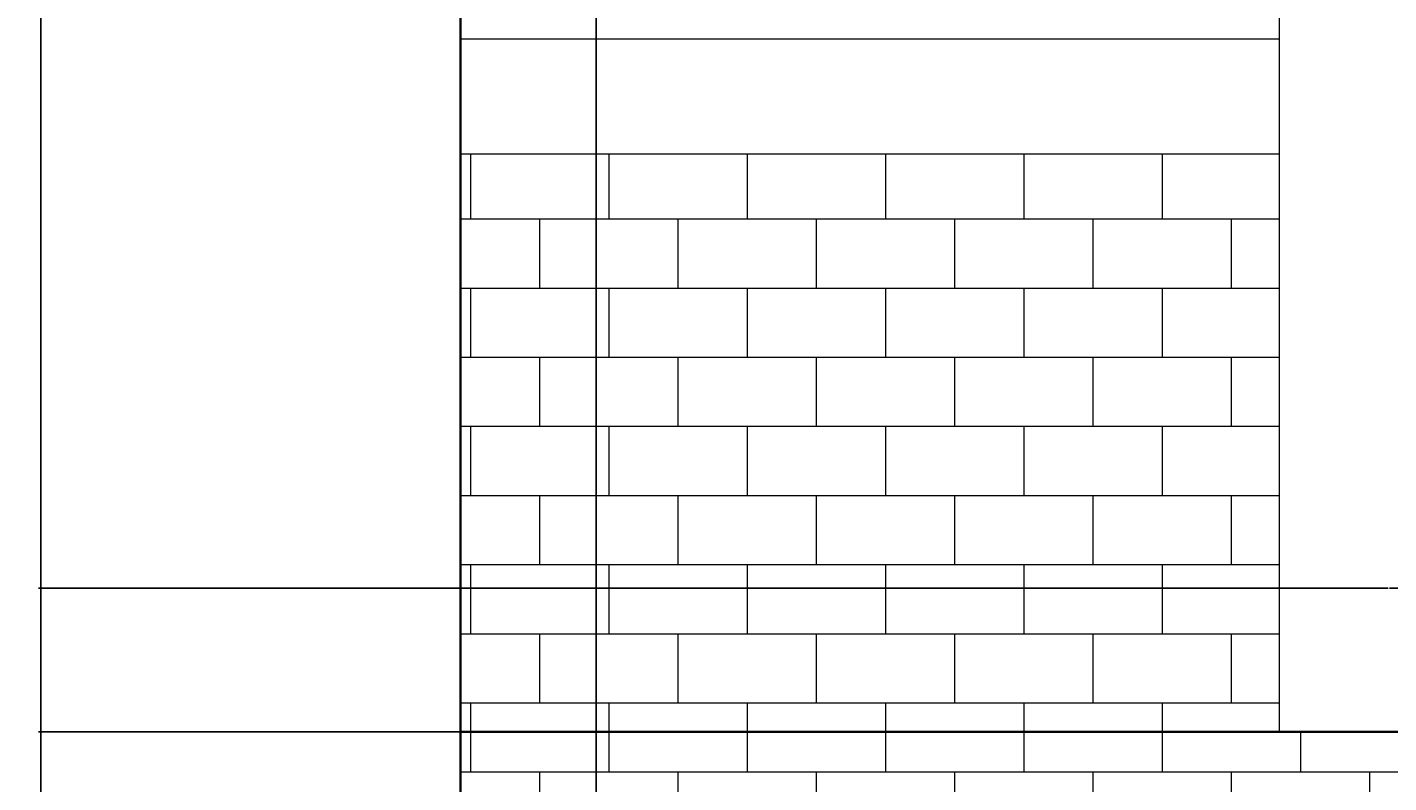
# Model space of a CAD drawing. Units: inches. Extents: x -26 to 776, y -22 to 650.
# Tile 7 of 62: x -26 to 92, y 155 to 221. Entities that reach past the tile are written whole.
import ezdxf

# ---------------------------------------------------------------- set-up
doc = ezdxf.new("R2010")
doc.units = ezdxf.units.IN
doc.header["$MEASUREMENT"] = 0
for name, color, linetype, lineweight in [('A-ANNO-DIMS', 2, 'Continuous', 18), ('A-WALL', 7, 'Continuous', 35), ('A-WALL-PATT', 8, 'Continuous', 13), ('A-WALL-TRIM', 7, 'Continuous', 18)]:
    doc.layers.add(name, color=color, linetype=linetype, lineweight=lineweight)
doc.styles.get("Standard").update_dxf_attribs({"font": 'arial.ttf'})
doc.dimstyles.get("Standard").update_dxf_attribs({"dimtxt": 0.5625, "dimasz": 0.18, "dimexe": 0.18, "dimexo": 0.0625, "dimgap": 0.09, "dimtad": 0, "dimtih": 1, "dimtoh": 1, "dimdec": 4, "dimzin": 0, "dimdsep": 46, "dimlunit": 4, "dimtxsty": 'Standard', "dimcen": 0.09, "dimadec": 0, "dimazin": 0, "dimtfac": 1, "dimtdec": 4, "dimtofl": 0, "dimtmove": 0, "dimatfit": 3, "dimfxl": 1, "dimtolj": 1, "dimtzin": 0, "dimarcsym": 0})

# ---------------------------------------------------------------- blocks, each defined once
blk = doc.blocks.new('*D14')
at = {"layer": 'A-ANNO-DIMS', "color": 0, "lineweight": -2, "transparency": 16777216}
for p, q in [((191.62, 613.27), (-25.48, 613.27)), ((-25.3, 613.09), (-25.3, 314.75)), ((-25.3, 15.66), (-25.3, 314)), ((11.04, 15.48), (-25.48, 15.48))]:
    blk.add_line(p, q, dxfattribs=at)
at = {"layer": 'A-ANNO-DIMS', "color": 0, "transparency": 16777216}
for points in [[(-25.33, 613.09), (-25.27, 613.09), (-25.3, 613.27)], [(-25.33, 15.66), (-25.27, 15.66), (-25.3, 15.48)]]:
    blk.add_solid(points, dxfattribs=at)
at = {"layer": 'Defpoints', "color": 0, "transparency": 16777216}
for p in [(-25.3, 613.27), (191.68, 613.27), (11.11, 15.48)]:
    blk.add_point(p, dxfattribs=at)
at = {"layer": 'A-ANNO-DIMS', "color": 0, "transparency": 16777216, "insert": (-25.3, 314.38), "char_height": 0.562, "attachment_point": 5}
blk.add_mtext('\\A1;597.8', dxfattribs=at)
blk = doc.blocks.new('*D22')
at = {"layer": 'A-ANNO-DIMS', "color": 0, "lineweight": -2, "transparency": 16777216}
for p, q in [((22.89, 15.33), (22.89, 649.86)), ((23.07, 649.68), (119.19, 649.68)), ((217.77, 649.68), (121.65, 649.68)), ((217.95, 15.54), (217.95, 649.86))]:
    blk.add_line(p, q, dxfattribs=at)
at = {"layer": 'A-ANNO-DIMS', "color": 0, "transparency": 16777216}
for points in [[(23.07, 649.71), (23.07, 649.65), (22.89, 649.68)], [(217.77, 649.71), (217.77, 649.65), (217.95, 649.68)]]:
    blk.add_solid(points, dxfattribs=at)
at = {"layer": 'Defpoints', "color": 0, "transparency": 16777216}
for p in [(217.95, 649.68), (217.95, 15.48), (22.89, 15.27)]:
    blk.add_point(p, dxfattribs=at)
at = {"layer": 'A-ANNO-DIMS', "color": 0, "transparency": 16777216, "insert": (120.42, 649.68), "char_height": 0.562, "attachment_point": 5}
blk.add_mtext('\\A1;195.06', dxfattribs=at)
blk = doc.blocks.new('*D24')
at = {"layer": 'A-ANNO-DIMS', "color": 0, "lineweight": -2, "transparency": 16777216}
for p, q in [((11.11, 15.54), (11.11, 649.86)), ((11.29, 649.68), (15.77, 649.68)), ((22.71, 649.68), (18.23, 649.68)), ((22.89, 15.33), (22.89, 649.86))]:
    blk.add_line(p, q, dxfattribs=at)
at = {"layer": 'A-ANNO-DIMS', "color": 0, "transparency": 16777216}
for points in [[(11.29, 649.71), (11.29, 649.65), (11.11, 649.68)], [(22.71, 649.71), (22.71, 649.65), (22.89, 649.68)]]:
    blk.add_solid(points, dxfattribs=at)
at = {"layer": 'Defpoints', "color": 0, "transparency": 16777216}
for p in [(22.89, 649.68), (11.11, 15.48), (22.89, 15.27)]:
    blk.add_point(p, dxfattribs=at)
at = {"layer": 'A-ANNO-DIMS', "color": 0, "transparency": 16777216, "insert": (17, 649.68), "char_height": 0.562, "attachment_point": 5}
blk.add_mtext('\\A1;11.782', dxfattribs=at)
blk = doc.blocks.new('*D26')
at = {"layer": 'A-ANNO-DIMS', "color": 0, "lineweight": -2, "transparency": 16777216}
for p, q in [((91.71, 171.97), (775.34, 171.97)), ((775.16, 171.79), (775.16, 166.11)), ((775.16, 159.66), (775.16, 165.35)), ((82.2, 159.48), (775.34, 159.48))]:
    blk.add_line(p, q, dxfattribs=at)
at = {"layer": 'A-ANNO-DIMS', "color": 0, "transparency": 16777216}
for points in [[(775.13, 171.79), (775.19, 171.79), (775.16, 171.97)], [(775.13, 159.66), (775.19, 159.66), (775.16, 159.48)]]:
    blk.add_solid(points, dxfattribs=at)
at = {"layer": 'Defpoints', "color": 0, "transparency": 16777216}
for p in [(91.64, 171.97), (775.16, 171.97), (82.13, 159.48)]:
    blk.add_point(p, dxfattribs=at)
at = {"layer": 'A-ANNO-DIMS', "color": 0, "transparency": 16777216, "insert": (775.16, 165.73), "char_height": 0.562, "attachment_point": 5}
blk.add_mtext('\\A1;12.49', dxfattribs=at)
blk = doc.blocks.new('*D27')
at = {"layer": 'A-ANNO-DIMS', "color": 0, "lineweight": -2, "transparency": 16777216}
for p, q in [((91.58, 306.86), (-25.48, 306.86)), ((-25.3, 306.68), (-25.3, 239.79)), ((-25.3, 172.15), (-25.3, 239.04)), ((91.58, 171.97), (-25.48, 171.97))]:
    blk.add_line(p, q, dxfattribs=at)
at = {"layer": 'A-ANNO-DIMS', "color": 0, "transparency": 16777216}
for points in [[(-25.33, 306.68), (-25.27, 306.68), (-25.3, 306.86)], [(-25.33, 172.15), (-25.27, 172.15), (-25.3, 171.97)]]:
    blk.add_solid(points, dxfattribs=at)
at = {"layer": 'Defpoints', "color": 0, "transparency": 16777216}
for p in [(-25.3, 306.86), (91.64, 306.86), (91.64, 171.97)]:
    blk.add_point(p, dxfattribs=at)
at = {"layer": 'A-ANNO-DIMS', "color": 0, "transparency": 16777216, "insert": (-25.3, 239.41), "char_height": 0.562, "attachment_point": 5}
blk.add_mtext('\\A1;134.88', dxfattribs=at)
blk = doc.blocks.new('*D36')
at = {"layer": 'A-ANNO-DIMS', "color": 0, "lineweight": -2, "transparency": 16777216}
for p, q in [((82.07, 420.28), (-25.48, 420.28)), ((-25.3, 420.1), (-25.3, 290.26)), ((-25.3, 159.66), (-25.3, 289.5)), ((82.07, 159.48), (-25.48, 159.48))]:
    blk.add_line(p, q, dxfattribs=at)
at = {"layer": 'A-ANNO-DIMS', "color": 0, "transparency": 16777216}
for points in [[(-25.33, 420.1), (-25.27, 420.1), (-25.3, 420.28)], [(-25.33, 159.66), (-25.27, 159.66), (-25.3, 159.48)]]:
    blk.add_solid(points, dxfattribs=at)
at = {"layer": 'Defpoints', "color": 0, "transparency": 16777216}
for p in [(-25.3, 420.28), (82.13, 420.28), (82.13, 159.48)]:
    blk.add_point(p, dxfattribs=at)
at = {"layer": 'A-ANNO-DIMS', "color": 0, "transparency": 16777216, "insert": (-25.3, 289.88), "char_height": 0.562, "attachment_point": 5}
blk.add_mtext('\\A1;260.8', dxfattribs=at)
blk = doc.blocks.new('*D37')
at = {"layer": 'A-ANNO-DIMS', "color": 0, "lineweight": -2, "transparency": 16777216}
for p, q in [((231.36, 159.48), (-25.48, 159.48)), ((-25.3, 159.3), (-25.3, 87.85)), ((-25.3, 15.66), (-25.3, 87.11)), ((217.89, 15.48), (-25.48, 15.48))]:
    blk.add_line(p, q, dxfattribs=at)
at = {"layer": 'A-ANNO-DIMS', "color": 0, "transparency": 16777216}
for points in [[(-25.33, 159.3), (-25.27, 159.3), (-25.3, 159.48)], [(-25.33, 15.66), (-25.27, 15.66), (-25.3, 15.48)]]:
    blk.add_solid(points, dxfattribs=at)
at = {"layer": 'Defpoints', "color": 0, "transparency": 16777216}
for p in [(-25.3, 159.48), (231.42, 159.48), (217.95, 15.48)]:
    blk.add_point(p, dxfattribs=at)
at = {"layer": 'A-ANNO-DIMS', "color": 0, "transparency": 16777216, "insert": (-25.3, 87.48), "char_height": 0.562, "attachment_point": 5}
blk.add_mtext('\\A1;144', dxfattribs=at)
blk = doc.blocks.new('*D41')
at = {"layer": 'A-ANNO-DIMS', "color": 0, "lineweight": -2, "transparency": 16777216}
for p, q in [((11.17, 221.64), (775.34, 221.64)), ((775.16, 221.46), (775.16, 190.94)), ((775.16, 159.66), (775.16, 190.18)), ((11.17, 159.48), (775.34, 159.48))]:
    blk.add_line(p, q, dxfattribs=at)
at = {"layer": 'A-ANNO-DIMS', "color": 0, "transparency": 16777216}
for points in [[(775.13, 221.46), (775.19, 221.46), (775.16, 221.64)], [(775.13, 159.66), (775.19, 159.66), (775.16, 159.48)]]:
    blk.add_solid(points, dxfattribs=at)
at = {"layer": 'Defpoints', "color": 0, "transparency": 16777216}
for p in [(11.11, 221.64), (775.16, 221.64), (11.11, 159.48)]:
    blk.add_point(p, dxfattribs=at)
at = {"layer": 'A-ANNO-DIMS', "color": 0, "transparency": 16777216, "insert": (775.16, 190.56), "char_height": 0.562, "attachment_point": 5}
blk.add_mtext('\\A1;62.16', dxfattribs=at)

msp = doc.modelspace()

# ---------------------------------------------------------------- hatches: boundary and pattern name
at = {"layer": 'A-WALL-PATT'}
h = msp.add_hatch(dxfattribs=at)
h.set_pattern_fill('AR-B816', color=256, scale=0.75)
h.paths.add_polyline_path([(82.134, 209.6413), (11.1074, 209.6413), (11.1074, 159.4824), (82.134, 159.4824)])
h.paths.add_polyline_path([(231.4249, 209.6413), (209.091, 209.6413), (209.091, 159.4824), (214.1056, 159.4824), (214.1056, 199.3298), (231.4249, 199.3298)])
h.paths.add_polyline_path([(231.4249, 159.4824), (11.1074, 159.4824), (11.1074, 22.5014), (22.8891, 22.5014), (22.8891, 147.0781), (217.9529, 147.0781), (217.9529, 20.7937), (231.4249, 20.7937)])
h.paths.add_polyline_path([(285.0179, 152.3087), (280.6173, 144.8359), (280.6173, 26.4239), (240.1654, 26.4239), (240.1654, 144.8359), (231.4249, 159.4824), (231.4249, 20.7937), (285.0179, 20.7937)])

# ---------------------------------------------------------------- linework, layer by layer
at = {"layer": 'A-WALL'}
for p, q in [((11.1074, 159.4824), (11.1074, 338.1203)), ((11.1074, 15.4824), (11.1074, 159.4824)), ((11.1074, 159.4824), (231.4249, 159.4824))]:
    msp.add_line(p, q, dxfattribs=at)
at = {"layer": 'A-WALL-TRIM'}
for p, q in [((11.1074, 219.6413), (82.134, 219.6413)), ((11.1074, 209.6413), (82.134, 209.6413))]:
    msp.add_line(p, q, dxfattribs=at)
msp.add_lwpolyline([(82.134, 159.4824), (209.091, 159.4824), (209.091, 420.2783), (82.134, 420.2783)], close=True, dxfattribs=at)

# ---------------------------------------------------------------- dimensions: what is measured, and where the dimension line sits
at = {"layer": 'A-ANNO-DIMS'}
for base, p1, p2, override, picture, middle in [((22.8891, 649.6763), (11.1074, 15.4824), (22.8891, 15.2701), {"dimdec": 3, "dimlfac": 1, "dimrnd": 0, "dimzin": 0, "dimdsep": 46, "dimlunit": 2}, '*D24', (16.9982, 649.6763)), ((217.9529, 649.6763), (22.8891, 15.2701), (217.9529, 15.4824), {"dimdec": 2, "dimlfac": 1, "dimrnd": 0, "dimzin": 0, "dimdsep": 46, "dimlunit": 2}, '*D22', (120.421, 649.6763))]:
    dim = msp.add_linear_dim(base=base, p1=p1, p2=p2, dimstyle='Standard', override=override, dxfattribs=at)
    dim.commit()
    dim.dimension.update_dxf_attribs({"geometry": picture, "text_midpoint": middle})
for base, p1, p2, override, picture, middle in [((-25.2976, 613.2713), (11.1074, 15.4824), (191.6782, 613.2713), {"dimdec": 1, "dimlfac": 1, "dimrnd": 0, "dimzin": 0, "dimdsep": 46, "dimlunit": 2}, '*D14', (-25.2976, 314.3769)), ((-25.2976, 420.2783), (82.134, 159.4824), (82.134, 420.2783), {"dimdec": 1, "dimlfac": 1, "dimrnd": 0, "dimzin": 0, "dimdsep": 46, "dimlunit": 2}, '*D36', (-25.2976, 289.8803)), ((-25.2976, 306.8552), (91.6448, 171.9734), (91.6448, 306.8552), {"dimdec": 2, "dimlfac": 1, "dimrnd": 0, "dimzin": 0, "dimdsep": 46, "dimlunit": 2}, '*D27', (-25.2976, 239.4143)), ((775.1553, 221.6413), (11.1074, 159.4824), (11.1074, 221.6413), {"dimdec": 2, "dimlfac": 1, "dimrnd": 0, "dimzin": 0, "dimdsep": 46, "dimlunit": 2}, '*D41', (775.1553, 190.5618)), ((775.1553, 171.9734), (82.134, 159.4824), (91.6448, 171.9734), {"dimdec": 2, "dimlfac": 1, "dimrnd": 0, "dimzin": 0, "dimdsep": 46, "dimlunit": 2}, '*D26', (775.1553, 165.7279)), ((-25.2976, 159.4824), (217.9529, 15.4824), (231.4249, 159.4824), {"dimdec": 0, "dimlfac": 1, "dimrnd": 0, "dimzin": 0, "dimdsep": 46, "dimlunit": 2}, '*D37', (-25.2976, 87.4824))]:
    dim = msp.add_linear_dim(base=base, p1=p1, p2=p2, angle=90, dimstyle='Standard', override=override, dxfattribs=at)
    dim.commit()
    dim.dimension.update_dxf_attribs({"geometry": picture, "text_midpoint": middle})

doc.saveas('drawing.dxf')
